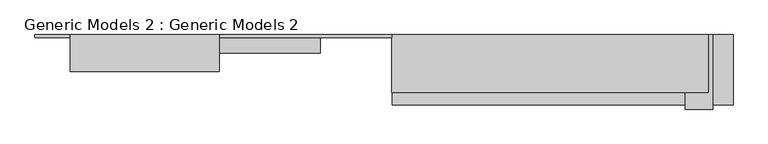
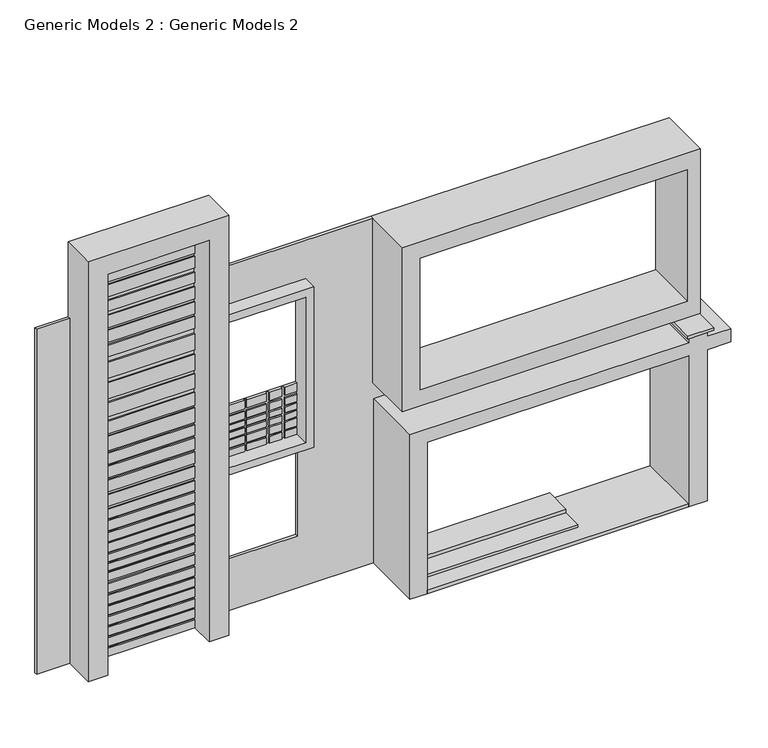
"""IFC4 building model written with IfcOpenShell, lengths in millimetres: proxy geometry, Generic Models 2 : Generic Models 2."""

from ifc_helpers import new_model, si_unit, frame, origin, origin_with_axes, place, context, project, spatial, polyline, outline, extrude, faceted_brep, source, transform, mapped, element, save


def generic_models_2_generic_models_2_25274e54(model_context):
    return source(origin(), model_context, "Body", "SolidModel", [
        faceted_brep([(-13682.3281629, -14899.7678064, 3807.1716172), (-13682.3281629, -14899.7678064, 3651.4774381), (-13412.4531629, -14899.7678064, 3651.4774381), (-13412.4531629, -14899.7678064, 3807.1716172), (-13682.3281629, -14899.7678064, 3600.2647557), (-13682.3281629, -14899.7678064, 3466.2078322), (-13412.4531629, -14899.7678064, 3466.2078322), (-13412.4531629, -14899.7678064, 3600.2647557), (-13682.3281629, -14899.7678064, 3435.6168773), (-13682.3281629, -14899.7678064, 3331.3341902), (-13412.4531629, -14899.7678064, 3331.3341902), (-13412.4531629, -14899.7678064, 3435.6168773), (-13682.3281629, -14899.7678064, 3296.5399023), (-13682.3281629, -14899.7678064, 3185.1594172), (-13412.4531629, -14899.7678064, 3185.1594172), (-13412.4531629, -14899.7678064, 3296.5399023), (-13682.3281629, -14899.7678064, 2983.1203976), (-13682.3281629, -14899.7678064, 2855.4967632), (-13412.4531629, -14899.7678064, 2855.4967632), (-13412.4531629, -14899.7678064, 2983.1203976), (-13682.3281629, -14899.7678064, 3156.6667349), (-13682.3281629, -14899.7678064, 3016.7935675), (-13412.4531629, -14899.7678064, 3016.7935675), (-13412.4531629, -14899.7678064, 3156.6667349), (-12158.3281629, -14899.7678064, 3651.4774381), (-12158.3281629, -14899.7678064, 3807.1716172), (-12378.3096317, -14899.7678064, 3807.1716172), (-12378.3096317, -14899.7678064, 3651.4774381), (-12158.3281629, -14899.7678064, 3466.2078322), (-12158.3281629, -14899.7678064, 3600.2647557), (-12378.3096317, -14899.7678064, 3600.2647557), (-12378.3096317, -14899.7678064, 3466.2078322), (-12158.3281629, -14899.7678064, 3331.3341902), (-12158.3281629, -14899.7678064, 3435.6168773), (-12378.3096317, -14899.7678064, 3435.6168773), (-12378.3096317, -14899.7678064, 3331.3341902), (-12158.3281629, -14899.7678064, 3185.1594172), (-12158.3281629, -14899.7678064, 3296.5399023), (-12378.3096317, -14899.7678064, 3296.5399023), (-12378.3096317, -14899.7678064, 3185.1594172), (-12158.3281629, -14899.7678064, 2855.4967632), (-12158.3281629, -14899.7678064, 2983.1203976), (-12378.3096317, -14899.7678064, 2983.1203976), (-12378.3096317, -14899.7678064, 2855.4967632), (-12158.3281629, -14899.7678064, 3016.7935675), (-12158.3281629, -14899.7678064, 3156.6667349), (-12378.3096317, -14899.7678064, 3156.6667349), (-12378.3096317, -14899.7678064, 3016.7935675), (-13080.557115, -14899.7678064, 3807.1716172), (-13371.7329008, -14899.7678064, 3807.1716172), (-13371.7329008, -14899.7678064, 3651.4774381), (-13080.557115, -14899.7678064, 3651.4774381), (-12698.0781629, -14899.7678064, 3807.1716172), (-13039.4499452, -14899.7678064, 3807.1716172), (-13039.4499452, -14899.7678064, 3651.4774381), (-12698.0781629, -14899.7678064, 3651.4774381), (-12428.2031629, -14899.7678064, 3807.1716172), (-12648.9318326, -14899.7678064, 3807.1716172), (-12648.9318326, -14899.7678064, 3651.4774381), (-12428.2031629, -14899.7678064, 3651.4774381), (-13371.7329008, -14899.7678064, 2855.4967632), (-13080.557115, -14899.7678064, 2855.4967632), (-13080.557115, -14899.7678064, 2983.1203976), (-13371.7329008, -14899.7678064, 2983.1203976), (-13039.4499452, -14899.7678064, 2855.4967632), (-12698.0781629, -14899.7678064, 2855.4967632), (-12698.0781629, -14899.7678064, 2983.1203976), (-13039.4499452, -14899.7678064, 2983.1203976), (-12648.9318326, -14899.7678064, 2855.4967632), (-12428.2031629, -14899.7678064, 2855.4967632), (-12428.2031629, -14899.7678064, 2983.1203976), (-12648.9318326, -14899.7678064, 2983.1203976), (-13371.7329008, -14899.7678064, 3466.2078322), (-13080.557115, -14899.7678064, 3466.2078322), (-13080.557115, -14899.7678064, 3600.2647557), (-13371.7329008, -14899.7678064, 3600.2647557), (-13039.4499452, -14899.7678064, 3466.2078322), (-12698.0781629, -14899.7678064, 3466.2078322), (-12698.0781629, -14899.7678064, 3600.2647557), (-13039.4499452, -14899.7678064, 3600.2647557), (-12648.9318326, -14899.7678064, 3466.2078322), (-12428.2031629, -14899.7678064, 3466.2078322), (-12428.2031629, -14899.7678064, 3600.2647557), (-12648.9318326, -14899.7678064, 3600.2647557), (-13371.7329008, -14899.7678064, 3331.3341902), (-13080.557115, -14899.7678064, 3331.3341902), (-13080.557115, -14899.7678064, 3435.6168773), (-13371.7329008, -14899.7678064, 3435.6168773), (-13039.4499452, -14899.7678064, 3331.3341902), (-12698.0781629, -14899.7678064, 3331.3341902), (-12698.0781629, -14899.7678064, 3435.6168773), (-13039.4499452, -14899.7678064, 3435.6168773), (-12648.9318326, -14899.7678064, 3331.3341902), (-12428.2031629, -14899.7678064, 3331.3341902), (-12428.2031629, -14899.7678064, 3435.6168773), (-12648.9318326, -14899.7678064, 3435.6168773), (-13371.7329008, -14899.7678064, 3185.1594172), (-13080.557115, -14899.7678064, 3185.1594172), (-13080.557115, -14899.7678064, 3296.5399023), (-13371.7329008, -14899.7678064, 3296.5399023), (-13039.4499452, -14899.7678064, 3185.1594172), (-12698.0781629, -14899.7678064, 3185.1594172), (-12698.0781629, -14899.7678064, 3296.5399023), (-13039.4499452, -14899.7678064, 3296.5399023), (-12648.9318326, -14899.7678064, 3185.1594172), (-12428.2031629, -14899.7678064, 3185.1594172), (-12428.2031629, -14899.7678064, 3296.5399023), (-12648.9318326, -14899.7678064, 3296.5399023), (-13371.7329008, -14899.7678064, 3016.7935675), (-13080.557115, -14899.7678064, 3016.7935675), (-13080.557115, -14899.7678064, 3156.6667349), (-13371.7329008, -14899.7678064, 3156.6667349), (-13039.4499452, -14899.7678064, 3016.7935675), (-12698.0781629, -14899.7678064, 3016.7935675), (-12698.0781629, -14899.7678064, 3156.6667349), (-13039.4499452, -14899.7678064, 3156.6667349), (-12648.9318326, -14899.7678064, 3016.7935675), (-12428.2031629, -14899.7678064, 3016.7935675), (-12428.2031629, -14899.7678064, 3156.6667349), (-12648.9318326, -14899.7678064, 3156.6667349), (-12158.3281629, -14848.9678064, 3807.1716172), (-12158.3281629, -14848.9678064, 2855.4967632), (-13682.3281629, -14848.9678064, 2855.4967632), (-13682.3281629, -14848.9678064, 3807.1716172), (-13412.4531629, -14874.3678064, 3807.1716172), (-13371.7329008, -14874.3678064, 3807.1716172), (-13080.557115, -14874.3678064, 3807.1716172), (-13039.4499452, -14874.3678064, 3807.1716172), (-12698.0781629, -14874.3678064, 3807.1716172), (-12648.9318326, -14874.3678064, 3807.1716172), (-12428.2031629, -14874.3678064, 3807.1716172), (-12378.3096317, -14874.3678064, 3807.1716172), (-13682.3281629, -14874.3678064, 2983.1203976), (-13682.3281629, -14874.3678064, 3016.7935675), (-13682.3281629, -14874.3678064, 3156.6667349), (-13682.3281629, -14874.3678064, 3185.1594172), (-13682.3281629, -14874.3678064, 3296.5399023), (-13682.3281629, -14874.3678064, 3331.3341902), (-13682.3281629, -14874.3678064, 3435.6168773), (-13682.3281629, -14874.3678064, 3466.2078322), (-13682.3281629, -14874.3678064, 3600.2647557), (-13682.3281629, -14874.3678064, 3651.4774381), (-12378.3096317, -14874.3678064, 2855.4967632), (-12428.2031629, -14874.3678064, 2855.4967632), (-12648.9318326, -14874.3678064, 2855.4967632), (-12698.0781629, -14874.3678064, 2855.4967632), (-13039.4499452, -14874.3678064, 2855.4967632), (-13080.557115, -14874.3678064, 2855.4967632), (-13371.7329008, -14874.3678064, 2855.4967632), (-13412.4531629, -14874.3678064, 2855.4967632), (-12158.3281629, -14874.3678064, 3651.4774381), (-12158.3281629, -14874.3678064, 3600.2647557), (-12158.3281629, -14874.3678064, 3466.2078322), (-12158.3281629, -14874.3678064, 3435.6168773), (-12158.3281629, -14874.3678064, 3331.3341902), (-12158.3281629, -14874.3678064, 3296.5399023), (-12158.3281629, -14874.3678064, 3185.1594172), (-12158.3281629, -14874.3678064, 3156.6667349), (-12158.3281629, -14874.3678064, 3016.7935675), (-12158.3281629, -14874.3678064, 2983.1203976), (-13412.4531629, -14874.3678064, 3600.2647557), (-13412.4531629, -14874.3678064, 3466.2078322), (-13412.4531629, -14874.3678064, 3435.6168773), (-13412.4531629, -14874.3678064, 3331.3341902), (-13412.4531629, -14874.3678064, 3296.5399023), (-13412.4531629, -14874.3678064, 3185.1594172), (-13412.4531629, -14874.3678064, 3156.6667349), (-13412.4531629, -14874.3678064, 3016.7935675), (-13412.4531629, -14874.3678064, 2983.1203976), (-13371.7329008, -14874.3678064, 2983.1203976), (-13080.557115, -14874.3678064, 2983.1203976), (-13039.4499452, -14874.3678064, 2983.1203976), (-12698.0781629, -14874.3678064, 2983.1203976), (-12648.9318326, -14874.3678064, 2983.1203976), (-12428.2031629, -14874.3678064, 2983.1203976), (-12378.3096317, -14874.3678064, 2983.1203976), (-12378.3096317, -14874.3678064, 3016.7935675), (-12378.3096317, -14874.3678064, 3156.6667349), (-12378.3096317, -14874.3678064, 3185.1594172), (-12378.3096317, -14874.3678064, 3296.5399023), (-12378.3096317, -14874.3678064, 3331.3341902), (-12378.3096317, -14874.3678064, 3435.6168773), (-12378.3096317, -14874.3678064, 3466.2078322), (-12378.3096317, -14874.3678064, 3600.2647557), (-12378.3096317, -14874.3678064, 3651.4774381), (-12428.2031629, -14874.3678064, 3651.4774381), (-12648.9318326, -14874.3678064, 3651.4774381), (-12698.0781629, -14874.3678064, 3651.4774381), (-13039.4499452, -14874.3678064, 3651.4774381), (-13080.557115, -14874.3678064, 3651.4774381), (-13371.7329008, -14874.3678064, 3651.4774381), (-13412.4531629, -14874.3678064, 3651.4774381), (-13371.7329008, -14874.3678064, 3600.2647557), (-13080.557115, -14874.3678064, 3600.2647557), (-13080.557115, -14874.3678064, 3466.2078322), (-13371.7329008, -14874.3678064, 3466.2078322), (-13039.4499452, -14874.3678064, 3600.2647557), (-12698.0781629, -14874.3678064, 3600.2647557), (-12698.0781629, -14874.3678064, 3466.2078322), (-13039.4499452, -14874.3678064, 3466.2078322), (-12648.9318326, -14874.3678064, 3600.2647557), (-12428.2031629, -14874.3678064, 3600.2647557), (-12428.2031629, -14874.3678064, 3466.2078322), (-12648.9318326, -14874.3678064, 3466.2078322), (-13371.7329008, -14874.3678064, 3435.6168773), (-13080.557115, -14874.3678064, 3435.6168773), (-13080.557115, -14874.3678064, 3331.3341902), (-13371.7329008, -14874.3678064, 3331.3341902), (-13039.4499452, -14874.3678064, 3435.6168773), (-12698.0781629, -14874.3678064, 3435.6168773), (-12698.0781629, -14874.3678064, 3331.3341902), (-13039.4499452, -14874.3678064, 3331.3341902), (-12648.9318326, -14874.3678064, 3435.6168773), (-12428.2031629, -14874.3678064, 3435.6168773), (-12428.2031629, -14874.3678064, 3331.3341902), (-12648.9318326, -14874.3678064, 3331.3341902), (-13371.7329008, -14874.3678064, 3296.5399023), (-13080.557115, -14874.3678064, 3296.5399023), (-13080.557115, -14874.3678064, 3185.1594172), (-13371.7329008, -14874.3678064, 3185.1594172), (-13039.4499452, -14874.3678064, 3296.5399023), (-12698.0781629, -14874.3678064, 3296.5399023), (-12698.0781629, -14874.3678064, 3185.1594172), (-13039.4499452, -14874.3678064, 3185.1594172), (-12648.9318326, -14874.3678064, 3296.5399023), (-12428.2031629, -14874.3678064, 3296.5399023), (-12428.2031629, -14874.3678064, 3185.1594172), (-12648.9318326, -14874.3678064, 3185.1594172), (-13371.7329008, -14874.3678064, 3156.6667349), (-13080.557115, -14874.3678064, 3156.6667349), (-13080.557115, -14874.3678064, 3016.7935675), (-13371.7329008, -14874.3678064, 3016.7935675), (-13039.4499452, -14874.3678064, 3156.6667349), (-12698.0781629, -14874.3678064, 3156.6667349), (-12698.0781629, -14874.3678064, 3016.7935675), (-13039.4499452, -14874.3678064, 3016.7935675), (-12648.9318326, -14874.3678064, 3156.6667349), (-12428.2031629, -14874.3678064, 3156.6667349), (-12428.2031629, -14874.3678064, 3016.7935675), (-12648.9318326, -14874.3678064, 3016.7935675)], [[[0, 1, 2, 3]], [[4, 5, 6, 7]], [[8, 9, 10, 11]], [[12, 13, 14, 15]], [[16, 17, 18, 19]], [[20, 21, 22, 23]], [[24, 25, 26, 27]], [[28, 29, 30, 31]], [[32, 33, 34, 35]], [[36, 37, 38, 39]], [[40, 41, 42, 43]], [[44, 45, 46, 47]], [[48, 49, 50, 51]], [[52, 53, 54, 55]], [[56, 57, 58, 59]], [[60, 61, 62, 63]], [[64, 65, 66, 67]], [[68, 69, 70, 71]], [[72, 73, 74, 75]], [[76, 77, 78, 79]], [[80, 81, 82, 83]], [[84, 85, 86, 87]], [[88, 89, 90, 91]], [[92, 93, 94, 95]], [[96, 97, 98, 99]], [[100, 101, 102, 103]], [[104, 105, 106, 107]], [[108, 109, 110, 111]], [[112, 113, 114, 115]], [[116, 117, 118, 119]], [[120, 121, 122, 123]], [[120, 123, 0, 3, 124, 125, 49, 48, 126, 127, 53, 52, 128, 129, 57, 56, 130, 131, 26, 25]], [[123, 122, 17, 16, 132, 133, 21, 20, 134, 135, 13, 12, 136, 137, 9, 8, 138, 139, 5, 4, 140, 141, 1, 0]], [[122, 121, 40, 43, 142, 143, 69, 68, 144, 145, 65, 64, 146, 147, 61, 60, 148, 149, 18, 17]], [[121, 120, 25, 24, 150, 151, 29, 28, 152, 153, 33, 32, 154, 155, 37, 36, 156, 157, 45, 44, 158, 159, 41, 40]], [[141, 140, 160, 161, 139, 138, 162, 163, 137, 136, 164, 165, 135, 134, 166, 167, 133, 132, 168, 149, 148, 169, 170, 147, 146, 171, 172, 145, 144, 173, 174, 143, 142, 175, 159, 158, 176, 177, 157, 156, 178, 179, 155, 154, 180, 181, 153, 152, 182, 183, 151, 150, 184, 131, 130, 185, 186, 129, 128, 187, 188, 127, 126, 189, 190, 125, 124, 191], [192, 193, 194, 195], [196, 197, 198, 199], [200, 201, 202, 203], [204, 205, 206, 207], [208, 209, 210, 211], [212, 213, 214, 215], [216, 217, 218, 219], [220, 221, 222, 223], [224, 225, 226, 227], [228, 229, 230, 231], [232, 233, 234, 235], [236, 237, 238, 239]], [[75, 74, 193, 192]], [[79, 78, 197, 196]], [[83, 82, 201, 200]], [[140, 4, 7, 160]], [[29, 151, 183, 30]], [[51, 50, 190, 189]], [[55, 54, 188, 187]], [[59, 58, 186, 185]], [[1, 141, 191, 2]], [[150, 24, 27, 184]], [[87, 86, 205, 204]], [[91, 90, 209, 208]], [[95, 94, 213, 212]], [[138, 8, 11, 162]], [[33, 153, 181, 34]], [[73, 72, 195, 194]], [[77, 76, 199, 198]], [[81, 80, 203, 202]], [[5, 139, 161, 6]], [[152, 28, 31, 182]], [[99, 98, 217, 216]], [[103, 102, 221, 220]], [[107, 106, 225, 224]], [[136, 12, 15, 164]], [[37, 155, 179, 38]], [[85, 84, 207, 206]], [[89, 88, 211, 210]], [[93, 92, 215, 214]], [[9, 137, 163, 10]], [[154, 32, 35, 180]], [[111, 110, 229, 228]], [[115, 114, 233, 232]], [[119, 118, 237, 236]], [[134, 20, 23, 166]], [[45, 157, 177, 46]], [[97, 96, 219, 218]], [[101, 100, 223, 222]], [[105, 104, 227, 226]], [[13, 135, 165, 14]], [[156, 36, 39, 178]], [[63, 62, 170, 169]], [[67, 66, 172, 171]], [[71, 70, 174, 173]], [[132, 16, 19, 168]], [[41, 159, 175, 42]], [[109, 108, 231, 230]], [[113, 112, 235, 234]], [[117, 116, 239, 238]], [[21, 133, 167, 22]], [[158, 44, 47, 176]], [[169, 148, 60, 63]], [[125, 190, 50, 49]], [[192, 195, 72, 75]], [[204, 207, 84, 87]], [[216, 219, 96, 99]], [[228, 231, 108, 111]], [[161, 160, 7, 6]], [[163, 162, 11, 10]], [[165, 164, 15, 14]], [[167, 166, 23, 22]], [[149, 168, 19, 18]], [[191, 124, 3, 2]], [[171, 146, 64, 67]], [[127, 188, 54, 53]], [[196, 199, 76, 79]], [[208, 211, 88, 91]], [[220, 223, 100, 103]], [[232, 235, 112, 115]], [[147, 170, 62, 61]], [[189, 126, 48, 51]], [[194, 193, 74, 73]], [[206, 205, 86, 85]], [[218, 217, 98, 97]], [[230, 229, 110, 109]], [[173, 144, 68, 71]], [[129, 186, 58, 57]], [[200, 203, 80, 83]], [[212, 215, 92, 95]], [[224, 227, 104, 107]], [[236, 239, 116, 119]], [[145, 172, 66, 65]], [[187, 128, 52, 55]], [[198, 197, 78, 77]], [[210, 209, 90, 89]], [[222, 221, 102, 101]], [[234, 233, 114, 113]], [[175, 142, 43, 42]], [[177, 176, 47, 46]], [[179, 178, 39, 38]], [[181, 180, 35, 34]], [[183, 182, 31, 30]], [[131, 184, 27, 26]], [[143, 174, 70, 69]], [[185, 130, 56, 59]], [[202, 201, 82, 81]], [[214, 213, 94, 93]], [[226, 225, 106, 105]], [[238, 237, 118, 117]]]),
        extrude(outline(polyline([(6400.8, -10834.6355238), (6400.8, -13682.3281629), (5692.341576, -13682.3281629), (5692.341576, -12017.3053381), (2721.859847, -12017.3053381), (2721.859847, -12158.3281629), (964.766173, -12158.3281629), (964.766173, -13682.3281629), (0.0, -13682.3281629), (0.0, -10821.3931635), (3048.0, -10821.3931635), (3048.0, -5605.1281629), (3352.8, -5605.1281629), (3352.8, -10821.3931635), (5692.341576, -10821.3931635), (5692.341576, -10834.6355238), (6400.8, -10834.6355238)])), frame((0.0, -14899.7678064, 0.0), z_axis=(0.0, 1.0, 0.0), x_axis=(0.0, 0.0, 1.0)), (0.0, 0.0, 1.0), 50.8),
        extrude(outline(polyline([(-16148.0386546, -14899.7678064), (-16730.3281629, -14899.7678064), (-16730.3281629, -14848.9678064), (-16148.0386546, -14848.9678064), (-16148.0386546, -14899.7678064)])), origin_with_axes(), (0.0, 0.0, 1.0), 6400.8),
        extrude(outline(polyline([(5692.341576, -12017.3053381), (5692.341576, -13682.3281629), (5552.8902612, -13682.3281629), (5552.8902612, -12158.3281629), (2855.4967632, -12158.3281629), (2855.4967632, -13682.3281629), (2721.859847, -13682.3281629), (2721.859847, -12017.3053381), (5692.341576, -12017.3053381)])), frame((0.0, -15153.7678064, 0.0), z_axis=(0.0, 1.0, 0.0), x_axis=(0.0, 0.0, 1.0)), (0.0, 0.0, 1.0), 304.8),
        faceted_brep([(-16148.0386546, -15458.5678064, 7792.3589427), (-16148.0386546, -15458.5678064, 0.0), (-15808.4178655, -15458.5678064, 0.0), (-15808.4178655, -15458.5678064, 7442.7838883), (-14025.2281629, -15458.5678064, 7442.7838883), (-14025.2281629, -15458.5678064, 0.0), (-13682.3281629, -15458.5678064, 0.0), (-13682.3281629, -15458.5678064, 7792.3589427), (-16148.0386546, -14848.9678064, 7792.3589427), (-13682.3281629, -14848.9678064, 7792.3589427), (-13682.3281629, -14848.9678064, 0.0), (-16148.0386546, -14848.9678064, 0.0), (-14025.2281629, -15026.7678064, 0.0), (-15808.4178655, -15026.7678064, 0.0), (-14025.2281629, -15026.7678064, 147.7434193), (-15808.4178655, -15026.7678064, 147.7434193), (-14025.2281629, -15026.7678064, 7442.7838883), (-15808.4178655, -15026.7678064, 7442.7838883), (-15808.4178655, -15026.7678064, 7202.5020592), (-14025.2281629, -15026.7678064, 7202.5020592), (-15808.4178655, -15026.7678064, 7139.4710655), (-15808.4178655, -15026.7678064, 6942.4992105), (-14025.2281629, -15026.7678064, 6942.4992105), (-14025.2281629, -15026.7678064, 7139.4710655), (-15808.4178655, -15026.7678064, 6887.347091), (-15808.4178655, -15026.7678064, 6670.6780505), (-14025.2281629, -15026.7678064, 6670.6780505), (-14025.2281629, -15026.7678064, 6887.347091), (-15808.4178655, -15026.7678064, 6591.8893084), (-15808.4178655, -15026.7678064, 6394.9174534), (-14025.2281629, -15026.7678064, 6394.9174534), (-14025.2281629, -15026.7678064, 6591.8893084), (-15808.4178655, -15026.7678064, 6320.0681484), (-15808.4178655, -15026.7678064, 6096.0), (-14025.2281629, -15026.7678064, 6096.0), (-14025.2281629, -15026.7678064, 6320.0681484), (-15808.4178655, -15026.7678064, 6041.5670733), (-15808.4178655, -15026.7678064, 5822.3288346), (-14025.2281629, -15026.7678064, 5822.3288346), (-14025.2281629, -15026.7678064, 6041.5670733), (-15808.4178655, -15026.7678064, 5770.9448724), (-15808.4178655, -15026.7678064, 5552.8902612), (-14025.2281629, -15026.7678064, 5552.8902612), (-14025.2281629, -15026.7678064, 5770.9448724), (-15808.4178655, -15026.7678064, 5454.1868633), (-15808.4178655, -15026.7678064, 5152.0123405), (-14025.2281629, -15026.7678064, 5152.0123405), (-14025.2281629, -15026.7678064, 5454.1868633), (-15808.4178655, -15026.7678064, 5068.6538514), (-15808.4178655, -15026.7678064, 4776.8991396), (-14025.2281629, -15026.7678064, 4776.8991396), (-14025.2281629, -15026.7678064, 5068.6538514), (-15808.4178655, -15026.7678064, 4703.9604617), (-15808.4178655, -15026.7678064, 4438.2552778), (-14025.2281629, -15026.7678064, 4438.2552778), (-14025.2281629, -15026.7678064, 4703.9604617), (-15808.4178655, -15026.7678064, 4360.1066943), (-15808.4178655, -15026.7678064, 4125.6609438), (-14025.2281629, -15026.7678064, 4125.6609438), (-14025.2281629, -15026.7678064, 4360.1066943), (-15808.4178655, -15026.7678064, 4076.1293734), (-15808.4178655, -15026.7678064, 3807.1716172), (-14025.2281629, -15026.7678064, 3807.1716172), (-14025.2281629, -15026.7678064, 4076.1293734), (-15808.4178655, -15026.7678064, 3763.8209258), (-15808.4178655, -15026.7678064, 3565.1677443), (-14025.2281629, -15026.7678064, 3565.1677443), (-14025.2281629, -15026.7678064, 3763.8209258), (-15808.4178655, -15026.7678064, 3523.8204702), (-15808.4178655, -15026.7678064, 3308.4993277), (-14025.2281629, -15026.7678064, 3308.4993277), (-14025.2281629, -15026.7678064, 3523.8204702), (-15808.4178655, -15026.7678064, 3263.3219136), (-15808.4178655, -15026.7678064, 3048.0), (-14025.2281629, -15026.7678064, 3048.0), (-14025.2281629, -15026.7678064, 3263.3219136), (-15808.4178655, -15026.7678064, 2991.1568063), (-15808.4178655, -15026.7678064, 2778.7697626), (-14025.2281629, -15026.7678064, 2778.7697626), (-14025.2281629, -15026.7678064, 2991.1568063), (-15808.4178655, -15026.7678064, 2721.859847), (-15808.4178655, -15026.7678064, 2550.7938638), (-14025.2281629, -15026.7678064, 2550.7938638), (-14025.2281629, -15026.7678064, 2721.859847), (-15808.4178655, -15026.7678064, 2513.8779131), (-15808.4178655, -15026.7678064, 2325.3881353), (-14025.2281629, -15026.7678064, 2325.3881353), (-14025.2281629, -15026.7678064, 2513.8779131), (-15808.4178655, -15026.7678064, 2289.7511945), (-15808.4178655, -15026.7678064, 2120.8222484), (-14025.2281629, -15026.7678064, 2120.8222484), (-14025.2281629, -15026.7678064, 2289.7511945), (-15808.4178655, -15026.7678064, 2091.541231), (-15808.4178655, -15026.7678064, 1929.3694427), (-14025.2281629, -15026.7678064, 1929.3694427), (-14025.2281629, -15026.7678064, 2091.541231), (-15808.4178655, -15026.7678064, 1895.5836535), (-15808.4178655, -15026.7678064, 1751.4309528), (-14025.2281629, -15026.7678064, 1751.4309528), (-14025.2281629, -15026.7678064, 1895.5836535), (-15808.4178655, -15026.7678064, 1715.3927776), (-15808.4178655, -15026.7678064, 1582.5020066), (-14025.2281629, -15026.7678064, 1582.5020066), (-14025.2281629, -15026.7678064, 1715.3927776), (-15808.4178655, -15026.7678064, 1546.4638315), (-15808.4178655, -15026.7678064, 1395.5539729), (-14025.2281629, -15026.7678064, 1395.5539729), (-14025.2281629, -15026.7678064, 1546.4638315), (-15808.4178655, -15026.7678064, 1348.253868), (-15808.4178655, -15026.7678064, 1176.0702241), (-14025.2281629, -15026.7678064, 1176.0702241), (-14025.2281629, -15026.7678064, 1348.253868), (-15808.4178655, -15026.7678064, 1132.0360788), (-15808.4178655, -15026.7678064, 964.766173), (-14025.2281629, -15026.7678064, 964.766173), (-14025.2281629, -15026.7678064, 1132.0360788), (-15808.4178655, -15026.7678064, 924.8165716), (-15808.4178655, -15026.7678064, 764.9931836), (-14025.2281629, -15026.7678064, 764.9931836), (-14025.2281629, -15026.7678064, 924.8165716), (-15808.4178655, -15026.7678064, 735.7287712), (-15808.4178655, -15026.7678064, 569.9531654), (-14025.2281629, -15026.7678064, 569.9531654), (-14025.2281629, -15026.7678064, 735.7287712), (-15808.4178655, -15026.7678064, 536.2799954), (-15808.4178655, -15026.7678064, 375.6848773), (-14025.2281629, -15026.7678064, 375.6848773), (-14025.2281629, -15026.7678064, 536.2799954), (-15808.4178655, -15026.7678064, 344.6019512), (-15808.4178655, -15026.7678064, 184.0068331), (-14025.2281629, -15026.7678064, 184.0068331), (-14025.2281629, -15026.7678064, 344.6019512), (-14025.2281629, -15001.3678064, 7202.5020592), (-14025.2281629, -15001.3678064, 7139.4710655), (-14025.2281629, -15001.3678064, 6942.4992105), (-14025.2281629, -15001.3678064, 6887.347091), (-14025.2281629, -15001.3678064, 6670.6780505), (-14025.2281629, -15001.3678064, 6591.8893084), (-14025.2281629, -15001.3678064, 6394.9174534), (-14025.2281629, -15001.3678064, 6320.0681484), (-14025.2281629, -15001.3678064, 6096.0), (-14025.2281629, -15001.3678064, 6041.5670733), (-14025.2281629, -15001.3678064, 5822.3288346), (-14025.2281629, -15001.3678064, 5770.9448724), (-14025.2281629, -15001.3678064, 5552.8902612), (-14025.2281629, -15001.3678064, 5454.1868633), (-14025.2281629, -15001.3678064, 5152.0123405), (-14025.2281629, -15001.3678064, 5068.6538514), (-14025.2281629, -15001.3678064, 4776.8991396), (-14025.2281629, -15001.3678064, 4703.9604617), (-14025.2281629, -15001.3678064, 4438.2552778), (-14025.2281629, -15001.3678064, 4360.1066943), (-14025.2281629, -15001.3678064, 4125.6609438), (-14025.2281629, -15001.3678064, 4076.1293734), (-14025.2281629, -15001.3678064, 3807.1716172), (-14025.2281629, -15001.3678064, 3763.8209258), (-14025.2281629, -15001.3678064, 3565.1677443), (-14025.2281629, -15001.3678064, 3523.8204702), (-14025.2281629, -15001.3678064, 3308.4993277), (-14025.2281629, -15001.3678064, 3263.3219136), (-14025.2281629, -15001.3678064, 3048.0), (-14025.2281629, -15001.3678064, 2991.1568063), (-14025.2281629, -15001.3678064, 2778.7697626), (-14025.2281629, -15001.3678064, 2721.859847), (-14025.2281629, -15001.3678064, 2550.7938638), (-14025.2281629, -15001.3678064, 2513.8779131), (-14025.2281629, -15001.3678064, 2325.3881353), (-14025.2281629, -15001.3678064, 2289.7511945), (-14025.2281629, -15001.3678064, 2120.8222484), (-14025.2281629, -15001.3678064, 2091.541231), (-14025.2281629, -15001.3678064, 1929.3694427), (-14025.2281629, -15001.3678064, 1895.5836535), (-14025.2281629, -15001.3678064, 1751.4309528), (-14025.2281629, -15001.3678064, 1715.3927776), (-14025.2281629, -15001.3678064, 1582.5020066), (-14025.2281629, -15001.3678064, 1546.4638315), (-14025.2281629, -15001.3678064, 1395.5539729), (-14025.2281629, -15001.3678064, 1348.253868), (-14025.2281629, -15001.3678064, 1176.0702241), (-14025.2281629, -15001.3678064, 1132.0360788), (-14025.2281629, -15001.3678064, 964.766173), (-14025.2281629, -15001.3678064, 924.8165716), (-14025.2281629, -15001.3678064, 764.9931836), (-14025.2281629, -15001.3678064, 735.7287712), (-14025.2281629, -15001.3678064, 569.9531654), (-14025.2281629, -15001.3678064, 536.2799954), (-14025.2281629, -15001.3678064, 375.6848773), (-14025.2281629, -15001.3678064, 344.6019512), (-14025.2281629, -15001.3678064, 184.0068331), (-14025.2281629, -15001.3678064, 147.7434193), (-15808.4178655, -15001.3678064, 147.7434193), (-15808.4178655, -15001.3678064, 184.0068331), (-15808.4178655, -15001.3678064, 344.6019512), (-15808.4178655, -15001.3678064, 375.6848773), (-15808.4178655, -15001.3678064, 536.2799954), (-15808.4178655, -15001.3678064, 569.9531654), (-15808.4178655, -15001.3678064, 735.7287712), (-15808.4178655, -15001.3678064, 764.9931836), (-15808.4178655, -15001.3678064, 924.8165716), (-15808.4178655, -15001.3678064, 964.766173), (-15808.4178655, -15001.3678064, 1132.0360788), (-15808.4178655, -15001.3678064, 1176.0702241), (-15808.4178655, -15001.3678064, 1348.253868), (-15808.4178655, -15001.3678064, 1395.5539729), (-15808.4178655, -15001.3678064, 1546.4638315), (-15808.4178655, -15001.3678064, 1582.5020066), (-15808.4178655, -15001.3678064, 1715.3927776), (-15808.4178655, -15001.3678064, 1751.4309528), (-15808.4178655, -15001.3678064, 1895.5836535), (-15808.4178655, -15001.3678064, 1929.3694427), (-15808.4178655, -15001.3678064, 2091.541231), (-15808.4178655, -15001.3678064, 2120.8222484), (-15808.4178655, -15001.3678064, 2289.7511945), (-15808.4178655, -15001.3678064, 2325.3881353), (-15808.4178655, -15001.3678064, 2513.8779131), (-15808.4178655, -15001.3678064, 2550.7938638), (-15808.4178655, -15001.3678064, 2721.859847), (-15808.4178655, -15001.3678064, 2778.7697626), (-15808.4178655, -15001.3678064, 2991.1568063), (-15808.4178655, -15001.3678064, 3048.0), (-15808.4178655, -15001.3678064, 3263.3219136), (-15808.4178655, -15001.3678064, 3308.4993277), (-15808.4178655, -15001.3678064, 3523.8204702), (-15808.4178655, -15001.3678064, 3565.1677443), (-15808.4178655, -15001.3678064, 3763.8209258), (-15808.4178655, -15001.3678064, 3807.1716172), (-15808.4178655, -15001.3678064, 4076.1293734), (-15808.4178655, -15001.3678064, 4125.6609438), (-15808.4178655, -15001.3678064, 4360.1066943), (-15808.4178655, -15001.3678064, 4438.2552778), (-15808.4178655, -15001.3678064, 4703.9604617), (-15808.4178655, -15001.3678064, 4776.8991396), (-15808.4178655, -15001.3678064, 5068.6538514), (-15808.4178655, -15001.3678064, 5152.0123405), (-15808.4178655, -15001.3678064, 5454.1868633), (-15808.4178655, -15001.3678064, 5552.8902612), (-15808.4178655, -15001.3678064, 5770.9448724), (-15808.4178655, -15001.3678064, 5822.3288346), (-15808.4178655, -15001.3678064, 6041.5670733), (-15808.4178655, -15001.3678064, 6096.0), (-15808.4178655, -15001.3678064, 6320.0681484), (-15808.4178655, -15001.3678064, 6394.9174534), (-15808.4178655, -15001.3678064, 6591.8893084), (-15808.4178655, -15001.3678064, 6670.6780505), (-15808.4178655, -15001.3678064, 6887.347091), (-15808.4178655, -15001.3678064, 6942.4992105), (-15808.4178655, -15001.3678064, 7139.4710655), (-15808.4178655, -15001.3678064, 7202.5020592)], [[[0, 1, 2, 3, 4, 5, 6, 7]], [[8, 9, 10, 11]], [[1, 0, 8, 11]], [[11, 10, 6, 5, 12, 13, 2, 1]], [[7, 6, 10, 9]], [[0, 7, 9, 8]], [[13, 12, 14, 15]], [[16, 17, 18, 19]], [[20, 21, 22, 23]], [[24, 25, 26, 27]], [[28, 29, 30, 31]], [[32, 33, 34, 35]], [[36, 37, 38, 39]], [[40, 41, 42, 43]], [[44, 45, 46, 47]], [[48, 49, 50, 51]], [[52, 53, 54, 55]], [[56, 57, 58, 59]], [[60, 61, 62, 63]], [[64, 65, 66, 67]], [[68, 69, 70, 71]], [[72, 73, 74, 75]], [[76, 77, 78, 79]], [[80, 81, 82, 83]], [[84, 85, 86, 87]], [[88, 89, 90, 91]], [[92, 93, 94, 95]], [[96, 97, 98, 99]], [[100, 101, 102, 103]], [[104, 105, 106, 107]], [[108, 109, 110, 111]], [[112, 113, 114, 115]], [[116, 117, 118, 119]], [[120, 121, 122, 123]], [[124, 125, 126, 127]], [[128, 129, 130, 131]], [[4, 16, 19, 132, 133, 23, 22, 134, 135, 27, 26, 136, 137, 31, 30, 138, 139, 35, 34, 140, 141, 39, 38, 142, 143, 43, 42, 144, 145, 47, 46, 146, 147, 51, 50, 148, 149, 55, 54, 150, 151, 59, 58, 152, 153, 63, 62, 154, 155, 67, 66, 156, 157, 71, 70, 158, 159, 75, 74, 160, 161, 79, 78, 162, 163, 83, 82, 164, 165, 87, 86, 166, 167, 91, 90, 168, 169, 95, 94, 170, 171, 99, 98, 172, 173, 103, 102, 174, 175, 107, 106, 176, 177, 111, 110, 178, 179, 115, 114, 180, 181, 119, 118, 182, 183, 123, 122, 184, 185, 127, 126, 186, 187, 131, 130, 188, 189, 14, 12, 5]], [[17, 3, 2, 13, 15, 190, 191, 129, 128, 192, 193, 125, 124, 194, 195, 121, 120, 196, 197, 117, 116, 198, 199, 113, 112, 200, 201, 109, 108, 202, 203, 105, 104, 204, 205, 101, 100, 206, 207, 97, 96, 208, 209, 93, 92, 210, 211, 89, 88, 212, 213, 85, 84, 214, 215, 81, 80, 216, 217, 77, 76, 218, 219, 73, 72, 220, 221, 69, 68, 222, 223, 65, 64, 224, 225, 61, 60, 226, 227, 57, 56, 228, 229, 53, 52, 230, 231, 49, 48, 232, 233, 45, 44, 234, 235, 41, 40, 236, 237, 37, 36, 238, 239, 33, 32, 240, 241, 29, 28, 242, 243, 25, 24, 244, 245, 21, 20, 246, 247, 18]], [[17, 16, 4, 3]], [[132, 247, 246, 133]], [[134, 245, 244, 135]], [[136, 243, 242, 137]], [[138, 241, 240, 139]], [[140, 239, 238, 141]], [[142, 237, 236, 143]], [[144, 235, 234, 145]], [[146, 233, 232, 147]], [[148, 231, 230, 149]], [[150, 229, 228, 151]], [[152, 227, 226, 153]], [[154, 225, 224, 155]], [[156, 223, 222, 157]], [[158, 221, 220, 159]], [[160, 219, 218, 161]], [[162, 217, 216, 163]], [[164, 215, 214, 165]], [[166, 213, 212, 167]], [[168, 211, 210, 169]], [[170, 209, 208, 171]], [[172, 207, 206, 173]], [[174, 205, 204, 175]], [[176, 203, 202, 177]], [[178, 201, 200, 179]], [[180, 199, 198, 181]], [[182, 197, 196, 183]], [[184, 195, 194, 185]], [[186, 193, 192, 187]], [[188, 191, 190, 189]], [[133, 246, 20, 23]], [[247, 132, 19, 18]], [[135, 244, 24, 27]], [[245, 134, 22, 21]], [[137, 242, 28, 31]], [[243, 136, 26, 25]], [[139, 240, 32, 35]], [[241, 138, 30, 29]], [[141, 238, 36, 39]], [[239, 140, 34, 33]], [[143, 236, 40, 43]], [[237, 142, 38, 37]], [[145, 234, 44, 47]], [[235, 144, 42, 41]], [[147, 232, 48, 51]], [[233, 146, 46, 45]], [[149, 230, 52, 55]], [[231, 148, 50, 49]], [[151, 228, 56, 59]], [[229, 150, 54, 53]], [[153, 226, 60, 63]], [[227, 152, 58, 57]], [[155, 224, 64, 67]], [[225, 154, 62, 61]], [[157, 222, 68, 71]], [[223, 156, 66, 65]], [[159, 220, 72, 75]], [[221, 158, 70, 69]], [[161, 218, 76, 79]], [[219, 160, 74, 73]], [[163, 216, 80, 83]], [[217, 162, 78, 77]], [[165, 214, 84, 87]], [[215, 164, 82, 81]], [[167, 212, 88, 91]], [[213, 166, 86, 85]], [[169, 210, 92, 95]], [[211, 168, 90, 89]], [[171, 208, 96, 99]], [[209, 170, 94, 93]], [[173, 206, 100, 103]], [[207, 172, 98, 97]], [[175, 204, 104, 107]], [[205, 174, 102, 101]], [[177, 202, 108, 111]], [[203, 176, 106, 105]], [[179, 200, 112, 115]], [[201, 178, 110, 109]], [[181, 198, 116, 119]], [[199, 180, 114, 113]], [[183, 196, 120, 123]], [[197, 182, 118, 117]], [[185, 194, 124, 127]], [[195, 184, 122, 121]], [[187, 192, 128, 131]], [[193, 186, 126, 125]], [[189, 190, 15, 14]], [[191, 188, 130, 129]]]),
        extrude(outline(polyline([(6400.8, -5605.1281629), (6400.8, -10834.6355238), (3352.8, -10834.6355238), (3352.8, -5605.1281629), (6400.8, -5605.1281629)]), holes=[polyline([(6096.0, -10520.0281629), (6096.0, -5833.7281629), (3657.3409284, -5833.7281629), (3657.3409284, -10520.0281629), (6096.0, -10520.0281629)])]), frame((0.0, -15802.0596162, 0.0), z_axis=(0.0, 1.0, 0.0), x_axis=(0.0, 0.0, 1.0)), (0.0, 0.0, 1.0), 953.0918098),
        extrude(outline(polyline([(-5986.1281629, -14848.9678064), (-5529.7265479, -14848.9678064), (-5529.7265479, -16080.8678064), (-5986.1281629, -16080.8678064), (-5986.1281629, -14848.9678064)])), frame((0.0, 0.0, 3175.9272397), z_axis=(0.0, 0.0, 1.0), x_axis=(1.0, 0.0, 0.0)), (0.0, 0.0, 1.0), 50.8),
        extrude(outline(polyline([(2804.8396505, -5192.2840012), (3048.0, -5192.2840012), (3048.0, -5605.1281629), (3175.9272397, -5605.1281629), (3175.9272397, -5933.3019227), (3048.0, -5933.3019227), (3048.0, -10821.3931635), (0.0, -10821.3931635), (0.0, -10520.0281629), (2804.8396505, -10520.0281629), (2804.8396505, -5933.3019227), (0.0, -5933.3019227), (0.0, -5605.1281629), (2804.8396505, -5605.1281629), (2804.8396505, -5192.2840012)])), frame((0.0, -16010.8553961, 0.0), z_axis=(0.0, 1.0, 0.0), x_axis=(0.0, 0.0, 1.0)), (0.0, 0.0, 1.0), 1161.8875897),
        extrude(outline(polyline([(-5933.3019227, -14848.9678064), (-5933.3019227, -16010.8553961), (-10520.0281629, -16010.8553961), (-10520.0281629, -15706.0553961), (-7700.6281629, -15706.0553961), (-7700.6281629, -14848.9678064), (-5933.3019227, -14848.9678064)])), origin_with_axes(), (0.0, 0.0, 1.0), 57.5794745),
        extrude(outline(polyline([(-7700.6281629, -15706.0553961), (-10520.0281629, -15706.0553961), (-10520.0281629, -15340.7856456), (-7700.6281629, -15340.7856456), (-7700.6281629, -15706.0553961)])), origin_with_axes(), (0.0, 0.0, 1.0), 105.1252773),
        extrude(outline(polyline([(-7700.6281629, -15340.7856456), (-10520.0281629, -15340.7856456), (-10520.0281629, -14848.9678064), (-7700.6281629, -14848.9678064), (-7700.6281629, -15340.7856456)])), origin_with_axes(), (0.0, 0.0, 1.0), 174.593796),
    ])


if __name__ == "__main__":
    model = new_model("IFC4")
    model_context = context("Model", 3, world=origin())
    ifc_project = project(units=[si_unit("LENGTHUNIT", "METRE", prefix="MILLI")], contexts=[model_context])
    site = spatial("IfcSite", under=ifc_project)
    building = spatial("IfcBuilding", under=site)
    placement = place(None, origin())
    generic_models_2_generic_models_2_shape = generic_models_2_generic_models_2_25274e54(model_context)
    element("IfcBuildingElementProxy", 1, Name="Generic Models 2 : Generic Models 2", ObjectType="Generic Models 2 : Generic Models 2", at=placement, inside=building, context=model_context, shape_type="MappedRepresentation", body=[
        mapped(generic_models_2_generic_models_2_shape, transform((0.0, 0.0, 0.0), x_axis=(1.0, 0.0, 0.0), y_axis=(0.0, 1.0, 0.0), z_axis=(0.0, 0.0, 1.0))),
    ])
    save(model, "model.ifc")
